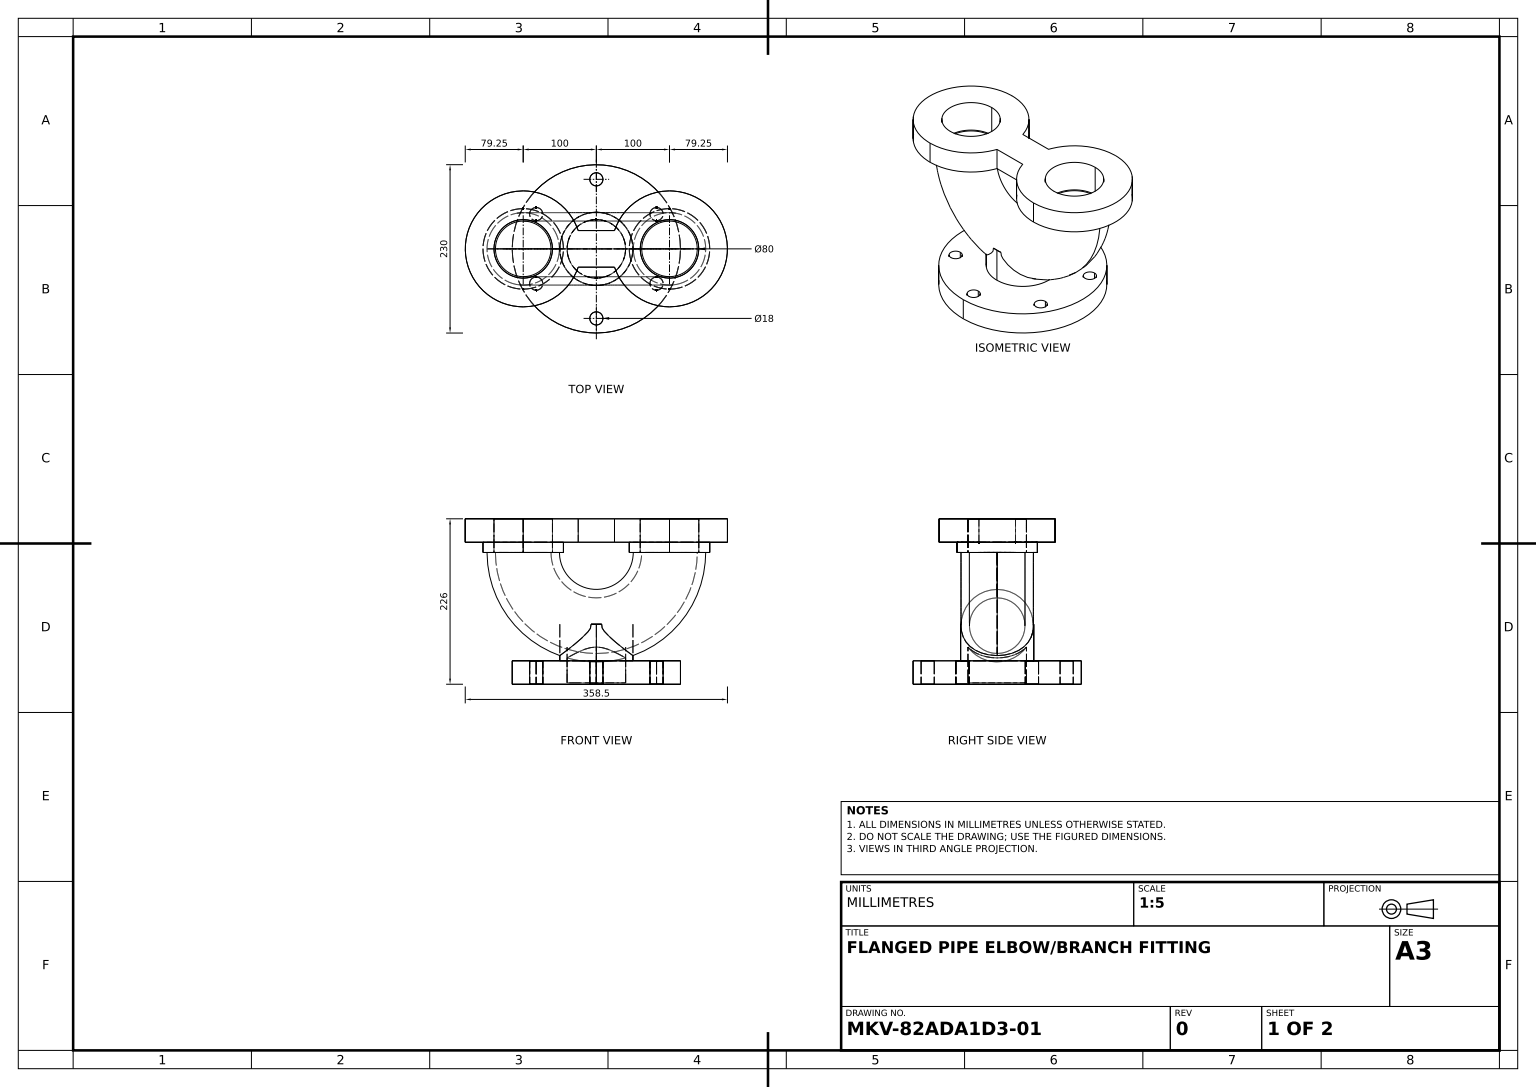
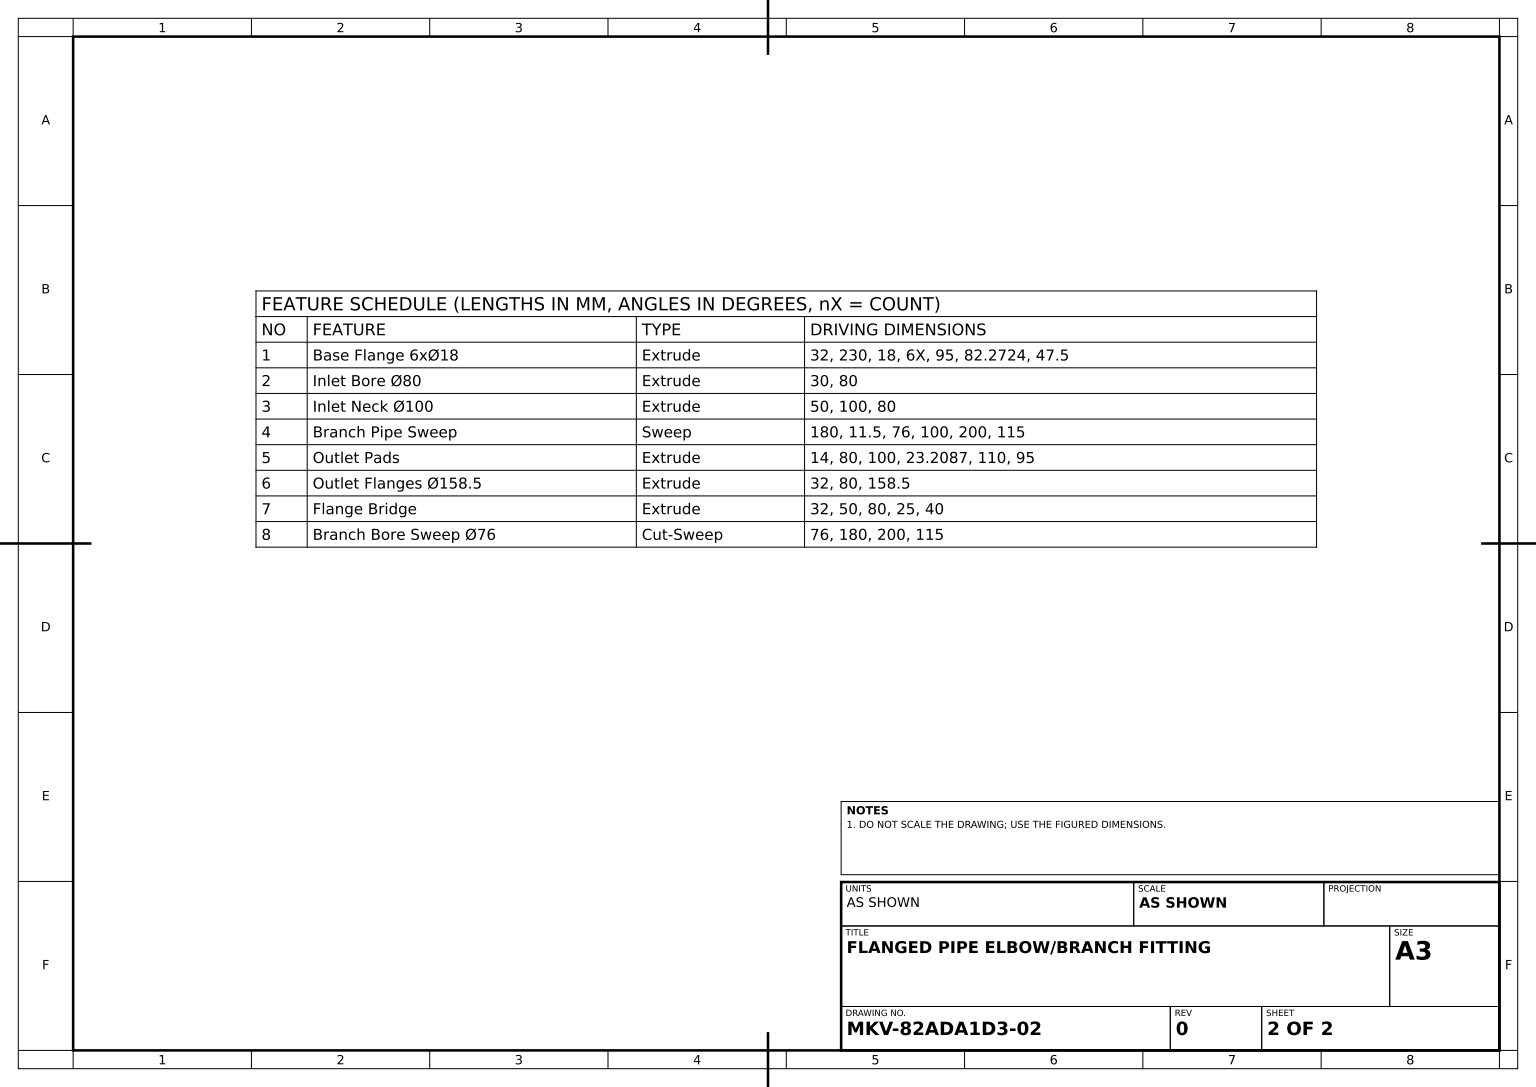
from build123d import *

# Parameters (mm, degrees)
BASE_FLANGE_SKETCH_R       = 115
BASE_FLANGE_SKETCH_R_2     = 9
BASE_FLANGE_6X_18_DEPTH    = 32
INLET_BORE_SKETCH_R        = 40
INLET_BORE_80_DEPTH        = 30
INLET_START                = 50
INLET_NECK_SKETCH_R        = 50
INLET_NECK_SKETCH_R_2      = 40
INLET_NECK_100_DEPTH       = 50
BRANCH_PROFILE_SKETCH_R    = 49.5
BRANCH_PROFILE_SKETCH_R_2  = 38
OUTLET_PAD_SKETCH_R        = 55
OUTLET_PAD_SKETCH_R_2      = 49.5
OUTLET_PAD_SKETCH_R_3      = 40
OUTLET_PADS_DEPTH          = 14
OUTLET_FLANGE_SKETCH_R     = 79.25
OUTLET_FLANGE_SKETCH_R_2   = 40
OUTLET_FLANGES_158_5_DEPTH = 32
FLANGE_BRIDGE_SKETCH_W     = 80
FLANGE_BRIDGE_SKETCH_H     = 50
FLANGE_BRIDGE_DEPTH        = 32
BRANCH_BORE_SKETCH_R       = 38


with BuildPart() as part:
    # Base Flange Sketch → Base Flange 6x_18 (new body)
    with BuildSketch(Plane(origin=(0, 0, 0), x_dir=(1, 0, 0), z_dir=(0, 1, 0))):
        with Locations(Location((0, 0, 0), (0, 0, 270))):
            Circle(BASE_FLANGE_SKETCH_R)
        with Locations(Location((0, 95, 0), (0, 0, 270))):
            Circle(BASE_FLANGE_SKETCH_R_2, mode=Mode.SUBTRACT)
        with Locations(Location((82.27241336, 47.5, 0), (0, 0, 270))):
            Circle(BASE_FLANGE_SKETCH_R_2, mode=Mode.SUBTRACT)
        with Locations(Location((82.27241336, -47.5, 0), (0, 0, 270))):
            Circle(BASE_FLANGE_SKETCH_R_2, mode=Mode.SUBTRACT)
        with Locations(Location((0, -95, 0), (0, 0, 270))):
            Circle(BASE_FLANGE_SKETCH_R_2, mode=Mode.SUBTRACT)
        with Locations(Location((-82.27241336, -47.5, 0), (0, 0, 270))):
            Circle(BASE_FLANGE_SKETCH_R_2, mode=Mode.SUBTRACT)
        with Locations(Location((-82.27241336, 47.5, 0), (0, 0, 270))):
            Circle(BASE_FLANGE_SKETCH_R_2, mode=Mode.SUBTRACT)
    extrude(amount=BASE_FLANGE_6X_18_DEPTH)

    # Inlet Bore Sketch → Inlet Bore _80 (cut)
    with BuildSketch(Plane(origin=(0, 32, 0), x_dir=(1, 0, 0), z_dir=(0, 1, 0))):
        with Locations(Location((0, 0, 0), (0, 0, 270))):
            Circle(INLET_BORE_SKETCH_R)
    extrude(amount=-INLET_BORE_80_DEPTH, mode=Mode.SUBTRACT)

    # Inlet Neck Sketch → Inlet Neck _100 (add)
    with BuildSketch(Plane(origin=(0, 32, 0), x_dir=(1, 0, 0), z_dir=(0, 1, 0)).offset(INLET_START)):
        with Locations(Location((0, 0, 0), (0, 0, 270))):
            Circle(INLET_NECK_SKETCH_R)
        with Locations(Location((0, 0, 0), (0, 0, 270))):
            Circle(INLET_NECK_SKETCH_R_2, mode=Mode.SUBTRACT)
    extrude(amount=-INLET_NECK_100_DEPTH)

    # Branch Pipe Sweep: sweep along a path in Branch Path Sketch
    with BuildLine(Plane.XY) as branch_pipe_sweep_path:
        ThreePointArc((-100, 180), (0, 80), (100, 180))
    # Branch Profile Sketch → Branch Pipe Sweep (sweep)
    with BuildSketch(Plane(origin=(0, 180, 0), x_dir=(1, 0, 0), z_dir=(0, 1, 0))):
        with Locations((100, 0)):
            Circle(BRANCH_PROFILE_SKETCH_R)
        with Locations((100, 0)):
            Circle(BRANCH_PROFILE_SKETCH_R_2, mode=Mode.SUBTRACT)
    sweep(path=branch_pipe_sweep_path.line)

    # Outlet Pad Sketch → Outlet Pads (add)
    # profile 1 of 3: a face of its own
    with BuildSketch(Plane(origin=(0, 180, 0), x_dir=(1, 0, 0), z_dir=(0, 1, 0))):
        with Locations(Location((-100, 0, 0), (0, 0, 270))):
            Circle(OUTLET_PAD_SKETCH_R)
        with Locations((-100, 0)):
            Circle(OUTLET_PAD_SKETCH_R_2, mode=Mode.SUBTRACT)
    # profile 2 of 3: a face of its own
    with BuildSketch(Plane(origin=(0, 180, 0), x_dir=(1, 0, 0), z_dir=(0, 1, 0))):
        with Locations((-100, 0)):
            Circle(OUTLET_PAD_SKETCH_R_2)
        with Locations(Location((-100, 0, 0), (0, 0, 270))):
            Circle(OUTLET_PAD_SKETCH_R_3, mode=Mode.SUBTRACT)
    # profile 3 of 3: a face of its own
    with BuildSketch(Plane(origin=(0, 180, 0), x_dir=(1, 0, 0), z_dir=(0, 1, 0))):
        with Locations(Location((100, 0, 0), (0, 0, 270))):
            Circle(OUTLET_PAD_SKETCH_R)
        with Locations(Location((100, 0, 0), (0, 0, 270))):
            Circle(OUTLET_PAD_SKETCH_R_3, mode=Mode.SUBTRACT)
    extrude(amount=OUTLET_PADS_DEPTH)

    # Outlet Flange Sketch → Outlet Flanges _158.5 (add)
    # profile 1 of 2: a face of its own
    with BuildSketch(Plane(origin=(0, 194, 0), x_dir=(1, 0, 0), z_dir=(0, 1, 0))):
        with Locations(Location((-100, 0, 0), (0, 0, 270))):
            Circle(OUTLET_FLANGE_SKETCH_R)
        with Locations(Location((-100, 0, 0), (0, 0, 270))):
            Circle(OUTLET_FLANGE_SKETCH_R_2, mode=Mode.SUBTRACT)
    # profile 2 of 2: a face of its own
    with BuildSketch(Plane(origin=(0, 194, 0), x_dir=(1, 0, 0), z_dir=(0, 1, 0))):
        with Locations(Location((100, 0, 0), (0, 0, 270))):
            Circle(OUTLET_FLANGE_SKETCH_R)
        with Locations(Location((100, 0, 0), (0, 0, 270))):
            Circle(OUTLET_FLANGE_SKETCH_R_2, mode=Mode.SUBTRACT)
    extrude(amount=OUTLET_FLANGES_158_5_DEPTH)

    # Flange Bridge Sketch → Flange Bridge (add)
    with BuildSketch(Plane(origin=(0, 226, 0), x_dir=(1, 0, 0), z_dir=(0, 1, 0))):
        Rectangle(FLANGE_BRIDGE_SKETCH_W, FLANGE_BRIDGE_SKETCH_H)
    extrude(amount=-FLANGE_BRIDGE_DEPTH)

    # Branch Bore Sweep _76: sweep along a path in Sketch7_2
    with BuildLine(Plane.XY) as branch_bore_sweep_76_path:
        ThreePointArc((-100, 180), (0, 80), (100, 180))
    # Branch Bore Sketch → Branch Bore Sweep _76 (sweep, cut)
    with BuildSketch(Plane(origin=(0, 180, 0), x_dir=(1, 0, 0), z_dir=(0, 1, 0))):
        with Locations((-100, 0)):
            Circle(BRANCH_BORE_SKETCH_R)
    sweep(path=branch_bore_sweep_76_path.line, mode=Mode.SUBTRACT)


solid = part.part
